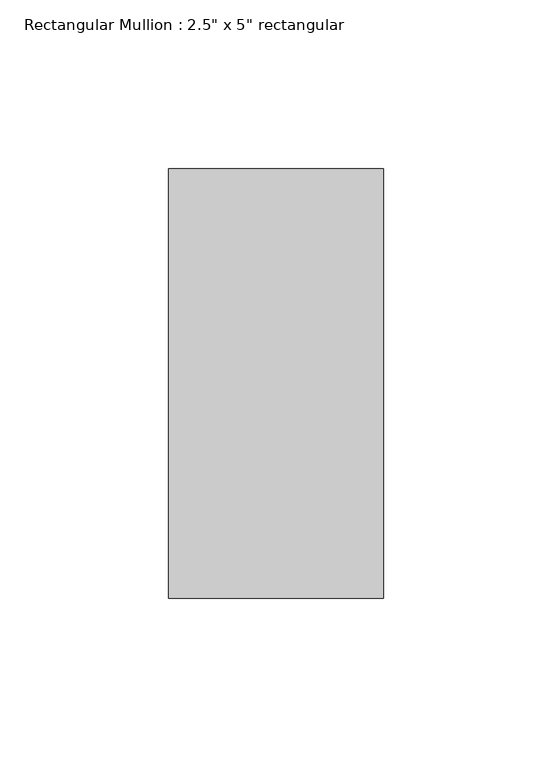
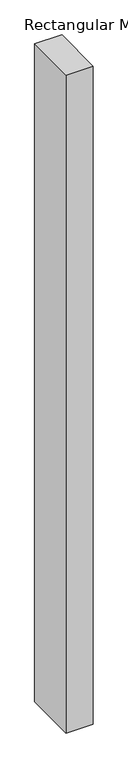
"""IFC4 building model written with IfcOpenShell, lengths in millimetres: member geometry."""

from ifc_helpers import new_model, si_unit, frame, origin, place, context, project, spatial, polyline, outline, extrude, source, transform, mapped, element, save


def member_62f62403(model_context):
    return source(origin(), model_context, "Body", "SweptSolid", [
        extrude(outline(polyline([(0.0, 63.5), (0.0, -63.5), (-63.5, -63.5), (-63.5, 63.5), (0.0, 63.5)])), frame((0.0, 0.0, -1628.7655616), z_axis=(0.0, 0.0, 1.0), x_axis=(1.0, 0.0, 0.0)), (0.0, 0.0, 1.0), 1628.7655616),
    ])


if __name__ == "__main__":
    model = new_model("IFC4")
    model_context = context("Model", 3, world=origin())
    ifc_project = project(units=[si_unit("LENGTHUNIT", "METRE", prefix="MILLI")], contexts=[model_context])
    site = spatial("IfcSite", under=ifc_project)
    building = spatial("IfcBuilding", under=site)
    placement = place(None, origin())
    member_shape = member_62f62403(model_context)
    element("IfcMember", 1, ObjectType="Rectangular Mullion : 2.5\" x 5\" rectangular", at=placement, inside=building, context=model_context, shape_type="MappedRepresentation", body=[
        mapped(member_shape, transform((0.0, 0.0, 0.0), x_axis=(1.0, 0.0, 0.0), y_axis=(0.0, 1.0, 0.0), z_axis=(0.0, 0.0, 1.0))),
    ])
    save(model, "model.ifc")

# Revit data of these elements
# Type "Rectangular Mullion : 2.5\" x 5\" rectangular"
#   built-in parameter 1007304 = 0.416667 (stored number, unit not read)
#   built-in parameter 1007301 = 0.104167 (stored number, unit not read)
#   built-in parameter 1007300 = 0.104167 (stored number, unit not read)
# Element 1 (IfcMember, "Rectangular Mullion : 2.5\" x 5\" rectangular")
#   Materials on its faces: "Aluminum"
# Materials
#   "Aluminum": class "Metal", colour RGB 247 247 247, transparency 0, Description = "Aluminum 6061", Cost = 0
